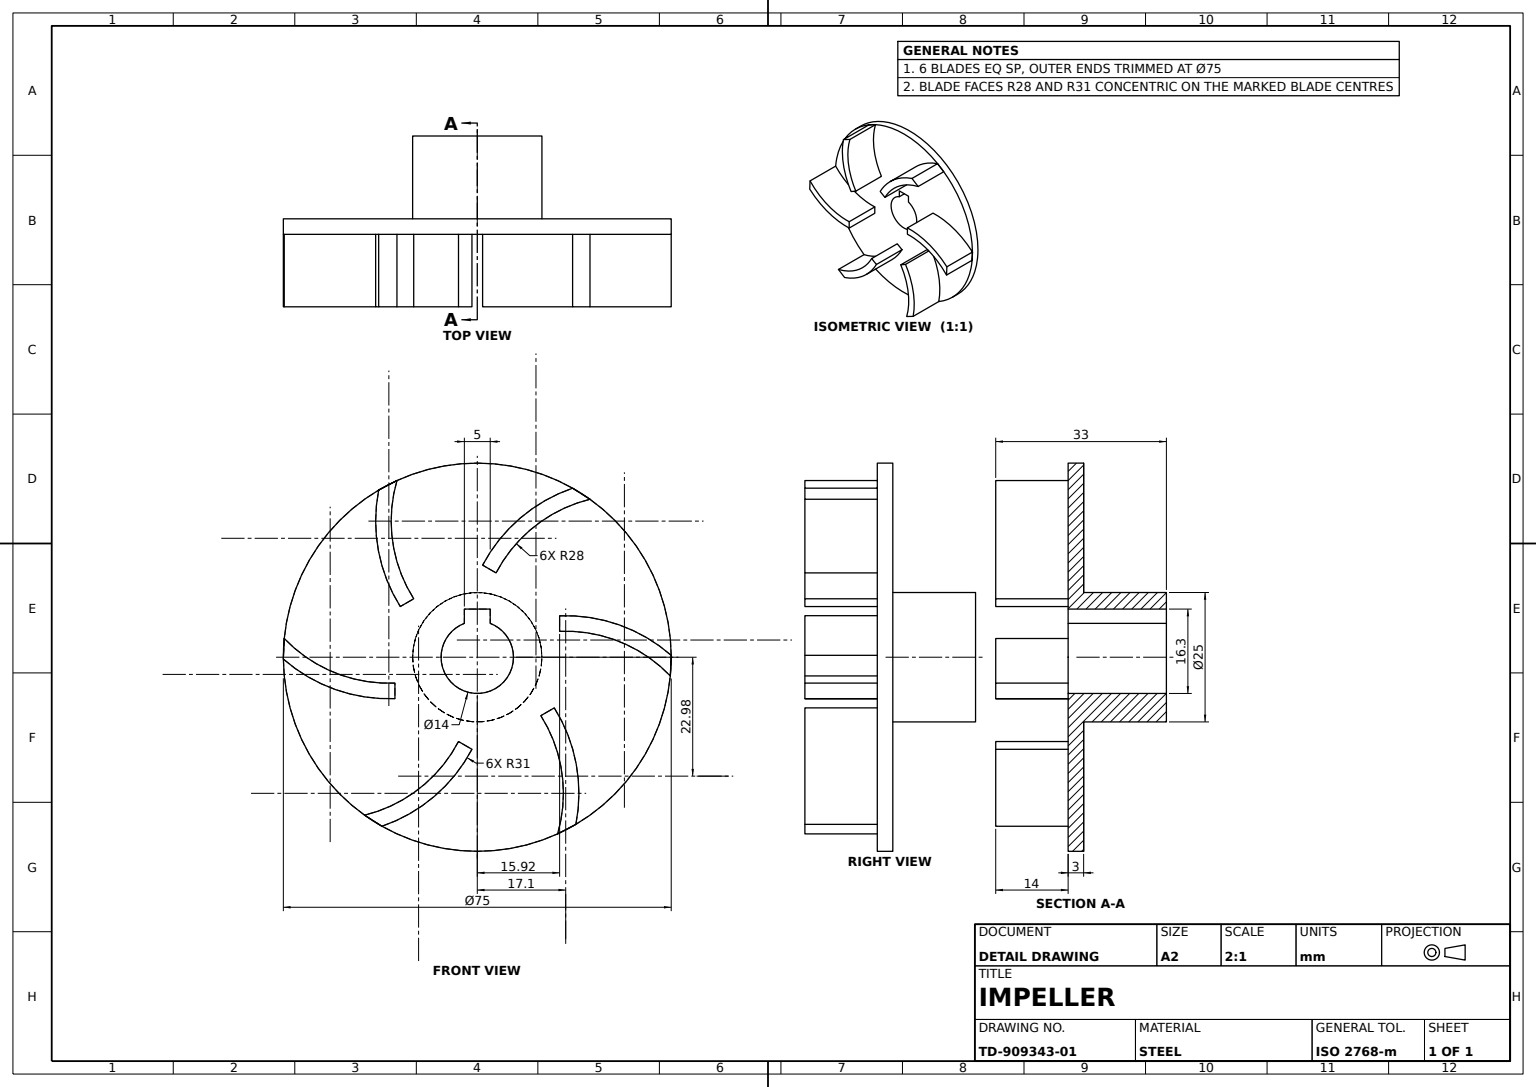
from build123d import *

# Parameters (mm, degrees)
BACK_DISC_SKETCH_R        = 37.5
BACK_DISC_75_DEPTH        = 3
BLADES_6X_DEPTH           = 14
HUB_SKETCH_R              = 12.5
HUB_25_DEPTH              = 16
KEYED_SHAFT_BORE_14_DEPTH = 63.461988441


with BuildPart() as part:
    # Back Disc Sketch → Back Disc Ø75 (new body)
    with BuildSketch(Plane.XY):
        Circle(BACK_DISC_SKETCH_R)
    extrude(amount=BACK_DISC_75_DEPTH)

    # Blade Profiles Sketch → Blades 6x (add)
    with BuildSketch(Plane.XY.offset(3)):
        with BuildLine():
            ThreePointArc((3.63084944, 16.288815705), (11.178007051, 25.36087614), (21.79252918, 30.51779271))
            Line((21.79252918, 30.51779271), (18.431665522, 32.657674536))
            ThreePointArc((18.431665522, 32.657674536), (8.308835539, 26.888544841), (1.030700016, 17.790012675))
            Line((1.030700016, 17.790012675), (3.63084944, 16.288815705))
        make_face()
        with BuildLine():
            ThreePointArc((-12.291103478, 11.288815705), (-16.374159474, 22.36087614), (-15.532919164, 34.131780238))
            Line((-15.532919164, 34.131780238), (-19.066543016, 32.291127844))
            ThreePointArc((-19.066543016, 32.291127844), (-19.131745134, 20.639935074), (-14.891252903, 9.787618735))
            Line((-14.891252903, 9.787618735), (-12.291103478, 11.288815705))
        make_face()
        with BuildLine():
            ThreePointArc((-15.921952918, -5), (-27.552166525, -3), (-37.325448345, 3.613987528))
            Line((-37.325448345, 3.613987528), (-37.498208538, -0.366546692))
            ThreePointArc((-37.498208538, -0.366546692), (-27.440580673, -6.248609768), (-15.921952918, -8.00239394))
            Line((-15.921952918, -8.00239394), (-15.921952918, -5))
        make_face()
        with BuildLine():
            ThreePointArc((-3.63084944, -16.288815705), (-11.178007051, -25.36087614), (-21.79252918, -30.51779271))
            Line((-21.79252918, -30.51779271), (-18.431665522, -32.657674536))
            ThreePointArc((-18.431665522, -32.657674536), (-8.308835539, -26.888544841), (-1.030700016, -17.790012675))
            Line((-1.030700016, -17.790012675), (-3.63084944, -16.288815705))
        make_face()
        with BuildLine():
            ThreePointArc((12.291103478, -11.288815705), (16.374159474, -22.36087614), (15.532919164, -34.131780238))
            Line((15.532919164, -34.131780238), (19.066543016, -32.291127844))
            ThreePointArc((19.066543016, -32.291127844), (19.131745134, -20.639935074), (14.891252903, -9.787618735))
            Line((14.891252903, -9.787618735), (12.291103478, -11.288815705))
        make_face()
        with BuildLine():
            ThreePointArc((15.921952918, 5), (27.552166525, 3), (37.325448345, -3.613987528))
            Line((37.325448345, -3.613987528), (37.498208538, 0.366546692))
            ThreePointArc((37.498208538, 0.366546692), (27.440580673, 6.248609768), (15.921952918, 8.00239394))
            Line((15.921952918, 8.00239394), (15.921952918, 5))
        make_face()
    extrude(amount=BLADES_6X_DEPTH)

    # Hub Sketch → Hub Ø25 (add)
    with BuildSketch(Plane(origin=(0, 0, 0), x_dir=(-1, 0, 0), z_dir=(0, 0, -1))):
        Circle(HUB_SKETCH_R)
    extrude(amount=HUB_25_DEPTH)

    # Shaft Bore Sketch → Keyed Shaft Bore Ø14 (cut, through all)
    with BuildSketch(Plane(origin=(0, 0, -16), x_dir=(-1, 0, 0), z_dir=(0, 0, -1))):
        with BuildLine():
            Line((-2.5, 6.538348415), (-2.5, 9.3))
            Line((-2.5, 9.3), (2.5, 9.3))
            Line((2.5, 9.3), (2.5, 6.538348415))
            ThreePointArc((2.5, 6.538348415), (0, -7), (-2.5, 6.538348415))
        make_face()
    extrude(amount=-KEYED_SHAFT_BORE_14_DEPTH, mode=Mode.SUBTRACT)


solid = part.part
